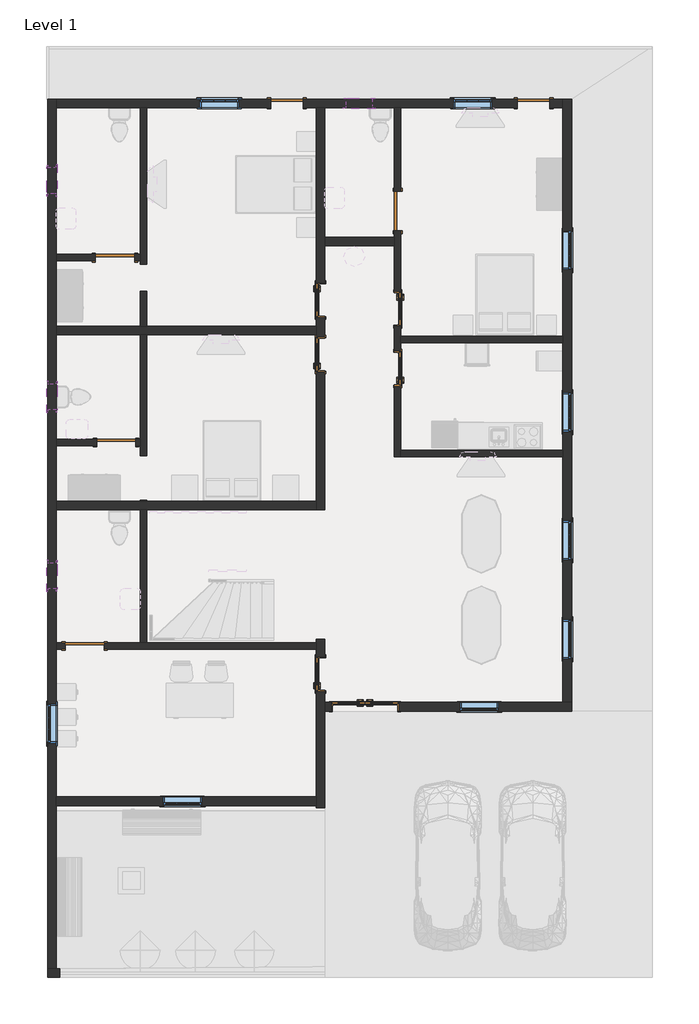
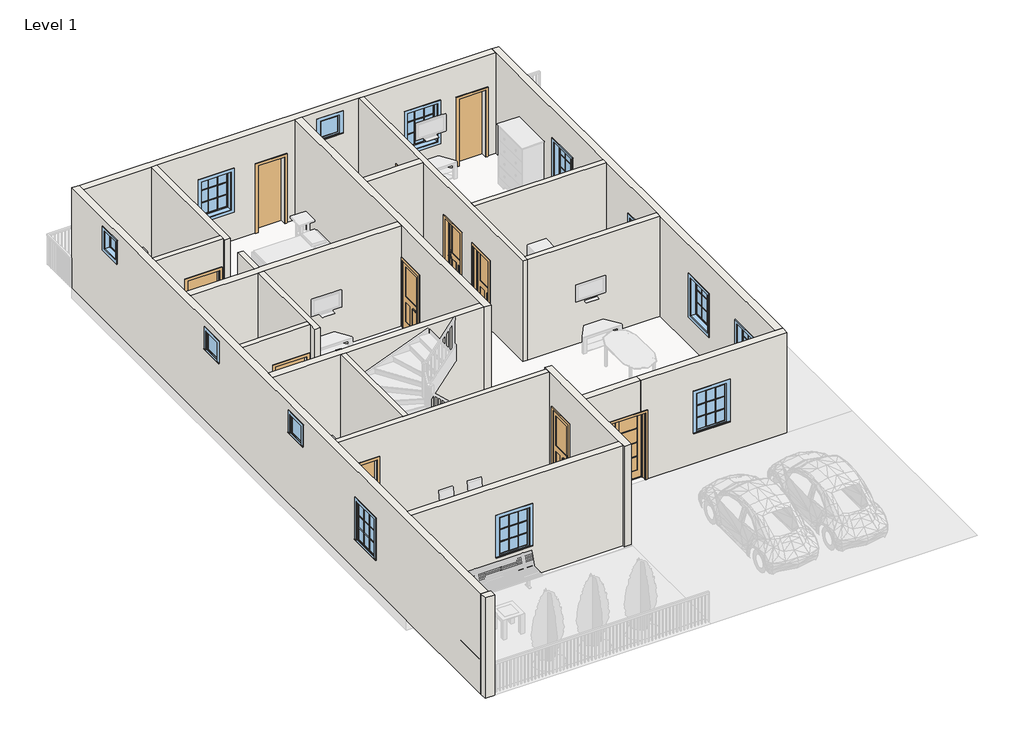
# One storey, part 1 of 4: 22 walls, 13 windows, 12 doors.
"""IFC4 building model written with IfcOpenShell, lengths in millimetres."""

from ifc_helpers import new_model, si_unit, frame, origin, origin_with_axes, place, context, project, spatial, polyline, outline, extrude, faceted_brep, transform, mapped, element, save
from components import door_7e6851c9, door_f50bbf81, door_cdf9d6cc, door_ce1fc124, door_b03bd389, door_fadea3f2, door_16372e1c, door_686f89d2, window_29c06734, window_e41d21a6

model = new_model("IFC4")

# Units and contexts
model_context = context("Model", 3, world=origin())
ifc_project = project(units=[si_unit("LENGTHUNIT", "METRE", prefix="MILLI")], contexts=[model_context])

# Site, building, storey
site = spatial("IfcSite", under=ifc_project)
building = spatial("IfcBuilding", under=site)
storey = spatial("IfcBuildingStorey", under=building, Name="Level 1", Elevation=0.0)

# Doors
placement = place(None, origin())
door_shape = door_7e6851c9(model_context)
element("IfcDoor", 1, ObjectType="30\" x 80\"", at=placement, inside=storey, context=model_context, shape_type="MappedRepresentation", body=[
    mapped(door_shape, transform((831.023647, -4225.8011892, 0.0), x_axis=(0.0, -1.0, 0.0), y_axis=(1.0, 0.0, 0.0), z_axis=(0.0, 0.0, 1.0))),
])
element("IfcDoor", 2, ObjectType="30\" x 80\"", at=placement, inside=storey, context=model_context, shape_type="MappedRepresentation", body=[
    mapped(door_shape, transform((831.023647, 3241.7988108, 0.0), x_axis=(0.0, -1.0, 0.0), y_axis=(1.0, 0.0, 0.0), z_axis=(0.0, 0.0, 1.0))),
])
door_2_shape = door_f50bbf81(model_context)
element("IfcDoor", 3, ObjectType="30\" x 80\"", at=placement, inside=storey, context=model_context, shape_type="MappedRepresentation", body=[
    mapped(door_2_shape, transform((831.023647, 4511.7988108, 0.0), x_axis=(0.0, 1.0, 0.0), y_axis=(-1.0, 0.0, 0.0), z_axis=(0.0, 0.0, 1.0))),
])
door_3_shape = door_cdf9d6cc(model_context)
element("IfcDoor", 4, ObjectType="30\" x 80\"", at=placement, inside=storey, context=model_context, shape_type="MappedRepresentation", body=[
    mapped(door_3_shape, transform((2640.773647, 2911.5988108, 0.0), x_axis=(0.0, -1.0, 0.0), y_axis=(1.0, 0.0, 0.0), z_axis=(0.0, 0.0, 1.0))),
])
door_4_shape = door_ce1fc124(model_context)
element("IfcDoor", 5, ObjectType="30\" x 80\"", at=placement, inside=storey, context=model_context, shape_type="MappedRepresentation", body=[
    mapped(door_4_shape, transform((2640.773647, 4308.5988108, 0.0), x_axis=(0.0, 1.0, 0.0), y_axis=(-1.0, 0.0, 0.0), z_axis=(0.0, 0.0, 1.0))),
])
door_5_shape = door_b03bd389(model_context)
element("IfcDoor", 6, ObjectType="Door-Exterior-Double-Full Glass-Wood_Clad : 60\" x 80\"", at=placement, inside=storey, context=model_context, shape_type="MappedRepresentation", body=[
    mapped(door_5_shape, transform((1875.598647, -4984.6261892, 0.0), x_axis=(1.0, 0.0, 0.0), y_axis=(0.0, 1.0, 0.0), z_axis=(0.0, 0.0, 1.0))),
])
door_6_shape = door_fadea3f2(model_context)
element("IfcDoor", 7, ObjectType="Single-Flush : 30\" x 80\"", at=placement, inside=storey, context=model_context, shape_type="MappedRepresentation", body=[
    mapped(door_6_shape, transform((46.798647, 9109.1988108, 0.0), x_axis=(1.0, 0.0, 0.0), y_axis=(0.0, 1.0, 0.0), z_axis=(0.0, 0.0, 1.0))),
])
element("IfcDoor", 8, ObjectType="Single-Flush : 30\" x 80\"", at=placement, inside=storey, context=model_context, shape_type="MappedRepresentation", body=[
    mapped(door_6_shape, transform((5812.598647, 9109.1988108, 0.0), x_axis=(1.0, 0.0, 0.0), y_axis=(0.0, 1.0, 0.0), z_axis=(0.0, 0.0, 1.0))),
])
door_7_shape = door_16372e1c(model_context)
element("IfcDoor", 9, ObjectType="Single-Flush : 36\" x 84\"", at=placement, inside=storey, context=model_context, shape_type="MappedRepresentation", body=[
    mapped(door_7_shape, transform((-3966.401353, 5502.3988108, 0.0), x_axis=(1.0, 0.0, 0.0), y_axis=(0.0, 1.0, 0.0), z_axis=(0.0, 0.0, 1.0))),
])
element("IfcDoor", 10, ObjectType="Single-Flush : 36\" x 84\"", at=placement, inside=storey, context=model_context, shape_type="MappedRepresentation", body=[
    mapped(door_7_shape, transform((-3941.001353, 1184.3988108, 0.0), x_axis=(1.0, 0.0, 0.0), y_axis=(0.0, 1.0, 0.0), z_axis=(0.0, 0.0, 1.0))),
])
door_8_shape = door_686f89d2(model_context)
element("IfcDoor", 11, ObjectType="Single-Flush : 36\" x 84\"", at=placement, inside=storey, context=model_context, shape_type="MappedRepresentation", body=[
    mapped(door_8_shape, transform((2637.598647, 6594.5988108, 0.0), x_axis=(0.0, -1.0, 0.0), y_axis=(1.0, 0.0, 0.0), z_axis=(0.0, 0.0, 1.0))),
])
element("IfcDoor", 12, ObjectType="Single-Flush : 36\" x 84\"", at=placement, inside=storey, context=model_context, shape_type="MappedRepresentation", body=[
    mapped(door_8_shape, transform((-4677.601353, -3565.4011892, 0.0), x_axis=(-1.0, 0.0, 0.0), y_axis=(0.0, -1.0, 0.0), z_axis=(0.0, 0.0, 1.0))),
])

# Walls
element("IfcWall", 13, ObjectType="Generic - 8\"", at=placement, inside=storey, context=model_context, shape_type="Brep", body=[
    faceted_brep([(-5338.001353, -11109.2011892, 0.0), (-5338.001353, -7299.2011892, 0.0), (-5338.001353, -7096.0011892, 0.0), (-5338.001353, -3641.6011892, 0.0), (-5338.001353, -3489.2011892, 0.0), (-5338.001353, -390.4011892, 0.0), (-5338.001353, -187.2011892, 0.0), (-5338.001353, 1108.1988108, 0.0), (-5338.001353, 1260.5988108, 0.0), (-5338.001353, 3698.9988108, 0.0), (-5338.001353, 3902.1988108, 0.0), (-5338.001353, 5426.1988108, 0.0), (-5338.001353, 5578.5988108, 0.0), (-5338.001353, 9007.5988108, 0.0), (-5338.001353, 9210.7988108, 0.0), (-5338.001353, 9210.7988108, 3048.0), (-5338.001353, 9007.5988108, 3048.0), (-5338.001353, 5578.5988108, 3048.0), (-5338.001353, 5426.1988108, 3048.0), (-5338.001353, 3902.1988108, 3048.0), (-5338.001353, 3698.9988108, 3048.0), (-5338.001353, 1260.5988108, 3048.0), (-5338.001353, 1108.1988108, 3048.0), (-5338.001353, -187.2011892, 3048.0), (-5338.001353, -390.4011892, 3048.0), (-5338.001353, -3489.2011892, 3048.0), (-5338.001353, -3641.6011892, 3048.0), (-5338.001353, -7096.0011892, 3048.0), (-5338.001353, -7299.2011892, 3048.0), (-5338.001353, -11109.2011892, 3048.0), (-5338.001353, -4924.3011892, 2133.6), (-5338.001353, -4924.3011892, 914.4), (-5338.001353, -5838.7011892, 914.4), (-5338.001353, -5838.7011892, 2133.6), (-5338.001353, -1622.3011892, 2768.6), (-5338.001353, -1622.3011892, 2159.0), (-5338.001353, -2231.9011892, 2159.0), (-5338.001353, -2231.9011892, 2768.6), (-5338.001353, 2555.9988108, 2768.6), (-5338.001353, 2555.9988108, 2159.0), (-5338.001353, 1946.3988108, 2159.0), (-5338.001353, 1946.3988108, 2768.6), (-5338.001353, 7000.9988108, 2768.6), (-5338.001353, 7610.5988108, 2768.6), (-5338.001353, 7610.5988108, 2159.0), (-5338.001353, 7000.9988108, 2159.0), (-5541.201353, -11109.2011892, 0.0), (-5541.201353, -11109.2011892, 3048.0), (-5541.201353, 9210.7988108, 3048.0), (-5541.201353, 9210.7988108, 0.0), (-5541.201353, -4924.3011892, 2133.6), (-5541.201353, -5838.7011892, 2133.6), (-5541.201353, -5838.7011892, 914.4), (-5541.201353, -4924.3011892, 914.4), (-5541.201353, -1622.3011892, 2768.6), (-5541.201353, -2231.9011892, 2768.6), (-5541.201353, -2231.9011892, 2159.0), (-5541.201353, -1622.3011892, 2159.0), (-5541.201353, 2555.9988108, 2768.6), (-5541.201353, 1946.3988108, 2768.6), (-5541.201353, 1946.3988108, 2159.0), (-5541.201353, 2555.9988108, 2159.0), (-5541.201353, 7000.9988108, 2768.6), (-5541.201353, 7000.9988108, 2159.0), (-5541.201353, 7610.5988108, 2159.0), (-5541.201353, 7610.5988108, 2768.6)], [[[0, 1, 2, 3, 4, 5, 6, 7, 8, 9, 10, 11, 12, 13, 14, 15, 16, 17, 18, 19, 20, 21, 22, 23, 24, 25, 26, 27, 28, 29], [30, 31, 32, 33], [34, 35, 36, 37], [38, 39, 40, 41], [42, 43, 44, 45]], [[46, 47, 48, 49], [50, 51, 52, 53], [54, 55, 56, 57], [58, 59, 60, 61], [62, 63, 64, 65]], [[14, 13, 12, 11, 10, 9, 8, 7, 6, 5, 4, 3, 2, 1, 0, 46, 49]], [[29, 28, 27, 26, 25, 24, 23, 22, 21, 20, 19, 18, 17, 16, 15, 48, 47]], [[0, 29, 47, 46]], [[15, 14, 49, 48]], [[31, 30, 50, 53]], [[32, 31, 53, 52]], [[33, 32, 52, 51]], [[30, 33, 51, 50]], [[35, 34, 54, 57]], [[36, 35, 57, 56]], [[37, 36, 56, 55]], [[34, 37, 55, 54]], [[39, 38, 58, 61]], [[40, 39, 61, 60]], [[41, 40, 60, 59]], [[38, 41, 59, 58]], [[63, 62, 42, 45]], [[64, 63, 45, 44]], [[65, 64, 44, 43]], [[62, 65, 43, 42]]]),
])
element("IfcWall", 14, ObjectType="Generic - 8\"", at=placement, inside=storey, context=model_context, shape_type="Brep", body=[
    faceted_brep([(6701.598647, -4886.2011892, 0.0), (6701.598647, 9210.7988108, 0.0), (6701.598647, 9210.7988108, 3048.0), (6701.598647, -4886.2011892, 3048.0), (6701.598647, 5222.9988108, 2133.6), (6701.598647, 6137.3988108, 2133.6), (6701.598647, 6137.3988108, 914.4), (6701.598647, 5222.9988108, 914.4), (6701.598647, 1438.3988108, 2133.6), (6701.598647, 2352.7988108, 2133.6), (6701.598647, 2352.7988108, 914.4), (6701.598647, 1438.3988108, 914.4), (6701.598647, -1558.8011892, 2133.6), (6701.598647, -644.4011892, 2133.6), (6701.598647, -644.4011892, 914.4), (6701.598647, -1558.8011892, 914.4), (6701.598647, -3870.2011892, 2133.6), (6701.598647, -2955.8011892, 2133.6), (6701.598647, -2955.8011892, 914.4), (6701.598647, -3870.2011892, 914.4), (6498.398647, -4886.2011892, 0.0), (6498.398647, -4886.2011892, 3048.0), (6498.398647, 854.1988108, 3048.0), (6498.398647, 1006.5988108, 3048.0), (6498.398647, 3521.1988108, 3048.0), (6498.398647, 3673.5988108, 3048.0), (6498.398647, 9007.5988108, 3048.0), (6498.398647, 9210.7988108, 3048.0), (6498.398647, 9210.7988108, 0.0), (6498.398647, 9007.5988108, 0.0), (6498.398647, 3673.5988108, 0.0), (6498.398647, 3521.1988108, 0.0), (6498.398647, 1006.5988108, 0.0), (6498.398647, 854.1988108, 0.0), (6498.398647, 5222.9988108, 2133.6), (6498.398647, 5222.9988108, 914.4), (6498.398647, 6137.3988108, 914.4), (6498.398647, 6137.3988108, 2133.6), (6498.398647, 1438.3988108, 2133.6), (6498.398647, 1438.3988108, 914.4), (6498.398647, 2352.7988108, 914.4), (6498.398647, 2352.7988108, 2133.6), (6498.398647, -1558.8011892, 2133.6), (6498.398647, -1558.8011892, 914.4), (6498.398647, -644.4011892, 914.4), (6498.398647, -644.4011892, 2133.6), (6498.398647, -3870.2011892, 2133.6), (6498.398647, -3870.2011892, 914.4), (6498.398647, -2955.8011892, 914.4), (6498.398647, -2955.8011892, 2133.6)], [[[0, 1, 2, 3], [4, 5, 6, 7], [8, 9, 10, 11], [12, 13, 14, 15], [16, 17, 18, 19]], [[20, 21, 22, 23, 24, 25, 26, 27, 28, 29, 30, 31, 32, 33], [34, 35, 36, 37], [38, 39, 40, 41], [42, 43, 44, 45], [46, 47, 48, 49]], [[1, 0, 20, 33, 32, 31, 30, 29, 28]], [[3, 2, 27, 26, 25, 24, 23, 22, 21]], [[2, 1, 28, 27]], [[0, 3, 21, 20]], [[35, 34, 4, 7]], [[36, 35, 7, 6]], [[37, 36, 6, 5]], [[34, 37, 5, 4]], [[39, 38, 8, 11]], [[40, 39, 11, 10]], [[41, 40, 10, 9]], [[38, 41, 9, 8]], [[43, 42, 12, 15]], [[44, 43, 15, 14]], [[45, 44, 14, 13]], [[42, 45, 13, 12]], [[47, 46, 16, 19]], [[48, 47, 19, 18]], [[49, 48, 18, 17]], [[46, 49, 17, 16]]]),
])
element("IfcWall", 15, ObjectType="Generic - 8\"", at=placement, inside=storey, context=model_context, shape_type="Brep", body=[
    faceted_brep([(6498.398647, 9210.7988108, 0.0), (6193.598647, 9210.7988108, 0.0), (6193.598647, 9210.7988108, 2032.0), (5431.598647, 9210.7988108, 2032.0), (5431.598647, 9210.7988108, 0.0), (427.798647, 9210.7988108, 0.0), (427.798647, 9210.7988108, 2032.0), (-334.201353, 9210.7988108, 2032.0), (-334.201353, 9210.7988108, 0.0), (-5338.001353, 9210.7988108, 0.0), (-5338.001353, 9210.7988108, 3048.0), (6498.398647, 9210.7988108, 3048.0), (-1070.801353, 9210.7988108, 2133.6), (-1985.201353, 9210.7988108, 2133.6), (-1985.201353, 9210.7988108, 914.4), (-1070.801353, 9210.7988108, 914.4), (4847.398647, 9210.7988108, 2133.6), (3932.998647, 9210.7988108, 2133.6), (3932.998647, 9210.7988108, 914.4), (4847.398647, 9210.7988108, 914.4), (1431.098647, 9210.7988108, 2768.6), (1431.098647, 9210.7988108, 2159.0), (2040.698647, 9210.7988108, 2159.0), (2040.698647, 9210.7988108, 2768.6), (6193.598647, 9007.5988108, 2032.0), (6193.598647, 9007.5988108, 0.0), (6498.398647, 9007.5988108, 0.0), (6498.398647, 9007.5988108, 3048.0), (2713.798647, 9007.5988108, 3048.0), (2561.398647, 9007.5988108, 3048.0), (935.798647, 9007.5988108, 3048.0), (732.598647, 9007.5988108, 3048.0), (-3229.801353, 9007.5988108, 3048.0), (-3382.201353, 9007.5988108, 3048.0), (-5338.001353, 9007.5988108, 3048.0), (-5338.001353, 9007.5988108, 0.0), (-3382.201353, 9007.5988108, 0.0), (-3229.801353, 9007.5988108, 0.0), (-334.201353, 9007.5988108, 0.0), (-334.201353, 9007.5988108, 2032.0), (427.798647, 9007.5988108, 2032.0), (427.798647, 9007.5988108, 0.0), (732.598647, 9007.5988108, 0.0), (935.798647, 9007.5988108, 0.0), (2561.398647, 9007.5988108, 0.0), (2713.798647, 9007.5988108, 0.0), (5431.598647, 9007.5988108, 0.0), (5431.598647, 9007.5988108, 2032.0), (-1070.801353, 9007.5988108, 2133.6), (-1070.801353, 9007.5988108, 914.4), (-1985.201353, 9007.5988108, 914.4), (-1985.201353, 9007.5988108, 2133.6), (4847.398647, 9007.5988108, 2133.6), (4847.398647, 9007.5988108, 914.4), (3932.998647, 9007.5988108, 914.4), (3932.998647, 9007.5988108, 2133.6), (1431.098647, 9007.5988108, 2768.6), (2040.698647, 9007.5988108, 2768.6), (2040.698647, 9007.5988108, 2159.0), (1431.098647, 9007.5988108, 2159.0)], [[[0, 1, 2, 3, 4, 5, 6, 7, 8, 9, 10, 11], [12, 13, 14, 15], [16, 17, 18, 19], [20, 21, 22, 23]], [[24, 25, 26, 27, 28, 29, 30, 31, 32, 33, 34, 35, 36, 37, 38, 39, 40, 41, 42, 43, 44, 45, 46, 47], [48, 49, 50, 51], [52, 53, 54, 55], [56, 57, 58, 59]], [[38, 37, 36, 35, 9, 8]], [[26, 25, 1, 0]], [[46, 45, 44, 43, 42, 41, 5, 4]], [[11, 10, 34, 33, 32, 31, 30, 29, 28, 27]], [[10, 9, 35, 34]], [[0, 11, 27, 26]], [[49, 48, 12, 15]], [[50, 49, 15, 14]], [[51, 50, 14, 13]], [[48, 51, 13, 12]], [[53, 52, 16, 19]], [[54, 53, 19, 18]], [[55, 54, 18, 17]], [[52, 55, 17, 16]], [[21, 20, 56, 59]], [[22, 21, 59, 58]], [[23, 22, 58, 57]], [[20, 23, 57, 56]], [[6, 5, 41, 40]], [[7, 6, 40, 39]], [[8, 7, 39, 38]], [[2, 1, 25, 24]], [[3, 2, 24, 47]], [[4, 3, 47, 46]]]),
])
element("IfcWall", 16, ObjectType="Generic - 8\"", at=placement, inside=storey, context=model_context, shape_type="SweptSolid", body=[
    extrude(outline(polyline([(0.0, -5338.001353), (0.0, 732.598647), (3048.0, 732.598647), (3048.0, -5338.001353), (0.0, -5338.001353)]), holes=[polyline([(2133.6, -2848.801353), (2133.6, -1934.401353), (914.4, -1934.401353), (914.4, -2848.801353), (2133.6, -2848.801353)])]), frame((0.0, -7299.2011892, 0.0), z_axis=(0.0, 1.0, 0.0), x_axis=(0.0, 0.0, 1.0)), (0.0, 0.0, 1.0), 203.2),
])
element("IfcWall", 17, ObjectType="Generic - 8\"", at=placement, inside=storey, context=model_context, shape_type="Brep", body=[
    faceted_brep([(935.798647, -3413.0011892, 0.0), (935.798647, -3413.0011892, 3048.0), (935.798647, -4886.2011892, 3048.0), (935.798647, -5089.4011892, 3048.0), (935.798647, -7350.0011892, 3048.0), (935.798647, -7350.0011892, 0.0), (935.798647, -5089.4011892, 0.0), (935.798647, -4886.2011892, 0.0), (935.798647, -4632.2011892, 0.0), (935.798647, -4632.2011892, 2057.4), (935.798647, -3819.4011892, 2057.4), (935.798647, -3819.4011892, 0.0), (732.598647, -3413.0011892, 3048.0), (732.598647, -3413.0011892, 0.0), (732.598647, -3489.2011892, 0.0), (732.598647, -3641.6011892, 0.0), (732.598647, -3819.4011892, 0.0), (732.598647, -3819.4011892, 2057.4), (732.598647, -4632.2011892, 2057.4), (732.598647, -4632.2011892, 0.0), (732.598647, -7096.0011892, 0.0), (732.598647, -7299.2011892, 0.0), (732.598647, -7350.0011892, 0.0), (732.598647, -7350.0011892, 3048.0), (732.598647, -7299.2011892, 3048.0), (732.598647, -7096.0011892, 3048.0), (732.598647, -3641.6011892, 3048.0), (732.598647, -3489.2011892, 3048.0)], [[[0, 1, 2, 3, 4, 5, 6, 7, 8, 9, 10, 11]], [[12, 13, 14, 15, 16, 17, 18, 19, 20, 21, 22, 23, 24, 25, 26, 27]], [[13, 0, 11, 16, 15, 14]], [[5, 22, 21, 20, 19, 8, 7, 6]], [[1, 0, 13, 12]], [[4, 3, 2, 1, 12, 27, 26, 25, 24, 23]], [[5, 4, 23, 22]], [[18, 9, 8, 19]], [[9, 18, 17, 10]], [[10, 17, 16, 11]]]),
])
element("IfcWall", 18, ObjectType="Generic - 8\"", at=placement, inside=storey, context=model_context, shape_type="Brep", body=[
    faceted_brep([(732.598647, -187.2011892, 0.0), (-3229.801353, -187.2011892, 0.0), (-3382.201353, -187.2011892, 0.0), (-5338.001353, -187.2011892, 0.0), (-5338.001353, -187.2011892, 3048.0), (-3382.201353, -187.2011892, 3048.0), (-3229.801353, -187.2011892, 3048.0), (732.598647, -187.2011892, 3048.0), (732.598647, -390.4011892, 0.0), (732.598647, -390.4011892, 3048.0), (-3229.801353, -390.4011892, 3048.0), (-3382.201353, -390.4011892, 3048.0), (-5338.001353, -390.4011892, 3048.0), (-5338.001353, -390.4011892, 0.0), (-3382.201353, -390.4011892, 0.0), (-3229.801353, -390.4011892, 0.0)], [[[0, 1, 2, 3, 4, 5, 6, 7]], [[8, 9, 10, 11, 12, 13, 14, 15]], [[3, 2, 1, 0, 8, 15, 14, 13]], [[7, 6, 5, 4, 12, 11, 10, 9]], [[4, 3, 13, 12]], [[0, 7, 9, 8]]]),
])
element("IfcWall", 19, ObjectType="Generic - 8\"", at=placement, inside=storey, context=model_context, shape_type="Brep", body=[
    faceted_brep([(732.598647, 3902.1988108, 0.0), (-3229.801353, 3902.1988108, 0.0), (-3382.201353, 3902.1988108, 0.0), (-5338.001353, 3902.1988108, 0.0), (-5338.001353, 3902.1988108, 3048.0), (-3382.201353, 3902.1988108, 3048.0), (-3229.801353, 3902.1988108, 3048.0), (732.598647, 3902.1988108, 3048.0), (732.598647, 3698.9988108, 0.0), (732.598647, 3698.9988108, 3048.0), (-3229.801353, 3698.9988108, 3048.0), (-3382.201353, 3698.9988108, 3048.0), (-5338.001353, 3698.9988108, 3048.0), (-5338.001353, 3698.9988108, 0.0), (-3382.201353, 3698.9988108, 0.0), (-3229.801353, 3698.9988108, 0.0)], [[[0, 1, 2, 3, 4, 5, 6, 7]], [[8, 9, 10, 11, 12, 13, 14, 15]], [[3, 2, 1, 0, 8, 15, 14, 13]], [[7, 6, 5, 4, 12, 11, 10, 9]], [[4, 3, 13, 12]], [[0, 7, 9, 8]]]),
])
element("IfcWall", 20, ObjectType="Generic - 8\"", at=placement, inside=storey, context=model_context, shape_type="SweptSolid", body=[
    extrude(outline(polyline([(3048.0, 2510.598647), (3048.0, 935.798647), (0.0, 935.798647), (0.0, 1088.198647), (2057.4, 1088.198647), (2057.4, 2510.598647), (3048.0, 2510.598647)])), frame((0.0, -5089.4011892, 0.0), z_axis=(0.0, 1.0, 0.0), x_axis=(0.0, 0.0, 1.0)), (0.0, 0.0, 1.0), 203.2),
])
element("IfcWall", 21, ObjectType="Generic - 8\"", at=placement, inside=storey, context=model_context, shape_type="SweptSolid", body=[
    extrude(outline(polyline([(935.798647, 5984.9988108), (2561.398647, 5984.9988108), (2561.398647, 5781.7988108), (935.798647, 5781.7988108), (935.798647, 5984.9988108)])), origin_with_axes(), (0.0, 0.0, 1.0), 3048.0),
])
element("IfcWall", 22, ObjectType="Generic - 8\"", at=placement, inside=storey, context=model_context, shape_type="Brep", body=[
    faceted_brep([(2510.598647, -4886.2011892, 3048.0), (6498.398647, -4886.2011892, 3048.0), (6701.598647, -4886.2011892, 3048.0), (6701.598647, -4886.2011892, 0.0), (6498.398647, -4886.2011892, 0.0), (2662.998647, -4886.2011892, 0.0), (2662.998647, -4886.2011892, 2057.4), (2510.598647, -4886.2011892, 2057.4), (4085.398647, -4886.2011892, 2133.6), (4085.398647, -4886.2011892, 914.4), (4999.798647, -4886.2011892, 914.4), (4999.798647, -4886.2011892, 2133.6), (6701.598647, -5089.4011892, 3048.0), (2510.598647, -5089.4011892, 3048.0), (2510.598647, -5089.4011892, 2057.4), (2662.998647, -5089.4011892, 2057.4), (2662.998647, -5089.4011892, 0.0), (6701.598647, -5089.4011892, 0.0), (4085.398647, -5089.4011892, 2133.6), (4999.798647, -5089.4011892, 2133.6), (4999.798647, -5089.4011892, 914.4), (4085.398647, -5089.4011892, 914.4)], [[[0, 1, 2, 3, 4, 5, 6, 7], [8, 9, 10, 11]], [[12, 13, 14, 15, 16, 17], [18, 19, 20, 21]], [[3, 17, 16, 5, 4]], [[13, 0, 7, 14]], [[2, 1, 0, 13, 12]], [[3, 2, 12, 17]], [[15, 6, 5, 16]], [[6, 15, 14, 7]], [[9, 8, 18, 21]], [[10, 9, 21, 20]], [[11, 10, 20, 19]], [[8, 11, 19, 18]]]),
])
element("IfcWall", 23, ObjectType="Generic - 8\"", at=placement, inside=storey, context=model_context, shape_type="Brep", body=[
    faceted_brep([(935.798647, 9007.5988108, 3048.0), (935.798647, 5984.9988108, 3048.0), (935.798647, 5781.7988108, 3048.0), (935.798647, -390.4011892, 3048.0), (935.798647, -390.4011892, 0.0), (935.798647, 2835.3988108, 0.0), (935.798647, 2835.3988108, 2057.4), (935.798647, 3648.1988108, 2057.4), (935.798647, 3648.1988108, 0.0), (935.798647, 4105.3988108, 0.0), (935.798647, 4105.3988108, 2057.4), (935.798647, 4918.1988108, 2057.4), (935.798647, 4918.1988108, 0.0), (935.798647, 5781.7988108, 0.0), (935.798647, 5984.9988108, 0.0), (935.798647, 9007.5988108, 0.0), (732.598647, -390.4011892, 3048.0), (732.598647, -187.2011892, 3048.0), (732.598647, 3698.9988108, 3048.0), (732.598647, 3902.1988108, 3048.0), (732.598647, 9007.5988108, 3048.0), (732.598647, 9007.5988108, 0.0), (732.598647, 4918.1988108, 0.0), (732.598647, 4918.1988108, 2057.4), (732.598647, 4105.3988108, 2057.4), (732.598647, 4105.3988108, 0.0), (732.598647, 3902.1988108, 0.0), (732.598647, 3698.9988108, 0.0), (732.598647, 3648.1988108, 0.0), (732.598647, 3648.1988108, 2057.4), (732.598647, 2835.3988108, 2057.4), (732.598647, 2835.3988108, 0.0), (732.598647, -187.2011892, 0.0), (732.598647, -390.4011892, 0.0)], [[[0, 1, 2, 3, 4, 5, 6, 7, 8, 9, 10, 11, 12, 13, 14, 15]], [[16, 17, 18, 19, 20, 21, 22, 23, 24, 25, 26, 27, 28, 29, 30, 31, 32, 33]], [[21, 15, 14, 13, 12, 22]], [[4, 33, 32, 31, 5]], [[25, 9, 8, 28, 27, 26]], [[3, 2, 1, 0, 20, 19, 18, 17, 16]], [[0, 15, 21, 20]], [[4, 3, 16, 33]], [[11, 23, 22, 12]], [[23, 11, 10, 24]], [[24, 10, 9, 25]], [[30, 6, 5, 31]], [[6, 30, 29, 7]], [[7, 29, 28, 8]]]),
])
element("IfcWall", 24, ObjectType="Generic - 8\"", at=placement, inside=storey, context=model_context, shape_type="Brep", body=[
    faceted_brep([(-5261.801353, -11109.2011892, 0.0), (-5338.001353, -11109.2011892, 0.0), (-5541.201353, -11109.2011892, 0.0), (-5541.201353, -11109.2011892, 3048.0), (-5338.001353, -11109.2011892, 3048.0), (-5261.801353, -11109.2011892, 3048.0), (-5261.801353, -11312.4011892, 0.0), (-5261.801353, -11312.4011892, 3048.0), (-5541.201353, -11312.4011892, 3048.0), (-5541.201353, -11312.4011892, 0.0)], [[[0, 1, 2, 3, 4, 5]], [[6, 7, 8, 9]], [[2, 1, 0, 6, 9]], [[5, 4, 3, 8, 7]], [[0, 5, 7, 6]], [[3, 2, 9, 8]]]),
])
element("IfcWall", 25, ObjectType="Inner wall", at=placement, inside=storey, context=model_context, shape_type="Brep", body=[
    faceted_brep([(2561.398647, 854.1988108, 3048.0), (2561.398647, 5781.7988108, 3048.0), (2561.398647, 5984.9988108, 3048.0), (2561.398647, 9007.5988108, 3048.0), (2561.398647, 9007.5988108, 0.0), (2561.398647, 7051.7988108, 0.0), (2561.398647, 7051.7988108, 2133.6), (2561.398647, 6137.3988108, 2133.6), (2561.398647, 6137.3988108, 0.0), (2561.398647, 5984.9988108, 0.0), (2561.398647, 5781.7988108, 0.0), (2561.398647, 4714.9988108, 0.0), (2561.398647, 4714.9988108, 2057.4), (2561.398647, 3902.1988108, 2057.4), (2561.398647, 3902.1988108, 0.0), (2561.398647, 3317.9988108, 0.0), (2561.398647, 3317.9988108, 2057.4), (2561.398647, 2505.1988108, 2057.4), (2561.398647, 2505.1988108, 0.0), (2561.398647, 854.1988108, 0.0), (2713.798647, 9007.5988108, 3048.0), (2713.798647, 3673.5988108, 3048.0), (2713.798647, 3521.1988108, 3048.0), (2713.798647, 1006.5988108, 3048.0), (2713.798647, 854.1988108, 3048.0), (2713.798647, 854.1988108, 0.0), (2713.798647, 1006.5988108, 0.0), (2713.798647, 2505.1988108, 0.0), (2713.798647, 2505.1988108, 2057.4), (2713.798647, 3317.9988108, 2057.4), (2713.798647, 3317.9988108, 0.0), (2713.798647, 3521.1988108, 0.0), (2713.798647, 3673.5988108, 0.0), (2713.798647, 3902.1988108, 0.0), (2713.798647, 3902.1988108, 2057.4), (2713.798647, 4714.9988108, 2057.4), (2713.798647, 4714.9988108, 0.0), (2713.798647, 6137.3988108, 0.0), (2713.798647, 6137.3988108, 2133.6), (2713.798647, 7051.7988108, 2133.6), (2713.798647, 7051.7988108, 0.0), (2713.798647, 9007.5988108, 0.0)], [[[0, 1, 2, 3, 4, 5, 6, 7, 8, 9, 10, 11, 12, 13, 14, 15, 16, 17, 18, 19]], [[20, 21, 22, 23, 24, 25, 26, 27, 28, 29, 30, 31, 32, 33, 34, 35, 36, 37, 38, 39, 40, 41]], [[4, 41, 40, 5]], [[25, 19, 18, 27, 26]], [[8, 37, 36, 11, 10, 9]], [[30, 15, 14, 33, 32, 31]], [[3, 2, 1, 0, 24, 23, 22, 21, 20]], [[4, 3, 20, 41]], [[0, 19, 25, 24]], [[38, 37, 8, 7]], [[39, 38, 7, 6]], [[40, 39, 6, 5]], [[17, 28, 27, 18]], [[28, 17, 16, 29]], [[29, 16, 15, 30]], [[35, 12, 11, 36]], [[12, 35, 34, 13]], [[13, 34, 33, 14]]]),
])
element("IfcWall", 26, ObjectType="Inner wall", at=placement, inside=storey, context=model_context, shape_type="Brep", body=[
    faceted_brep([(-5134.801353, -3489.2011892, 2133.6), (-5134.801353, -3489.2011892, 0.0), (-5338.001353, -3489.2011892, 0.0), (-5338.001353, -3489.2011892, 3048.0), (-3382.201353, -3489.2011892, 3048.0), (-3229.801353, -3489.2011892, 3048.0), (732.598647, -3489.2011892, 3048.0), (732.598647, -3489.2011892, 0.0), (-3229.801353, -3489.2011892, 0.0), (-3382.201353, -3489.2011892, 0.0), (-4220.401353, -3489.2011892, 0.0), (-4220.401353, -3489.2011892, 2133.6), (-5338.001353, -3641.6011892, 0.0), (-5134.801353, -3641.6011892, 0.0), (-5134.801353, -3641.6011892, 2133.6), (-4220.401353, -3641.6011892, 2133.6), (-4220.401353, -3641.6011892, 0.0), (732.598647, -3641.6011892, 0.0), (732.598647, -3641.6011892, 3048.0), (-5338.001353, -3641.6011892, 3048.0)], [[[0, 1, 2, 3, 4, 5, 6, 7, 8, 9, 10, 11]], [[12, 13, 14, 15, 16, 17, 18, 19]], [[2, 1, 13, 12]], [[10, 9, 8, 7, 17, 16]], [[6, 5, 4, 3, 19, 18]], [[3, 2, 12, 19]], [[7, 6, 18, 17]], [[14, 13, 1, 0]], [[15, 14, 0, 11]], [[16, 15, 11, 10]]]),
])
element("IfcWall", 27, ObjectType="Inner wall", at=placement, inside=storey, context=model_context, shape_type="Brep", body=[
    faceted_brep([(-3382.201353, 9007.5988108, 0.0), (-3382.201353, 5578.5988108, 0.0), (-3382.201353, 5426.1988108, 0.0), (-3382.201353, 5349.9988108, 0.0), (-3382.201353, 5349.9988108, 3048.0), (-3382.201353, 5426.1988108, 3048.0), (-3382.201353, 5578.5988108, 3048.0), (-3382.201353, 9007.5988108, 3048.0), (-3229.801353, 9007.5988108, 0.0), (-3229.801353, 9007.5988108, 3048.0), (-3229.801353, 5349.9988108, 3048.0), (-3229.801353, 5349.9988108, 0.0)], [[[0, 1, 2, 3, 4, 5, 6, 7]], [[8, 9, 10, 11]], [[3, 2, 1, 0, 8, 11]], [[4, 3, 11, 10]], [[7, 6, 5, 4, 10, 9]], [[0, 7, 9, 8]]]),
])
element("IfcWall", 28, ObjectType="Inner wall", at=placement, inside=storey, context=model_context, shape_type="SweptSolid", body=[
    extrude(outline(polyline([(2713.798647, 1006.5988108), (6498.398647, 1006.5988108), (6498.398647, 854.1988108), (2713.798647, 854.1988108), (2713.798647, 1006.5988108)])), origin_with_axes(), (0.0, 0.0, 1.0), 3048.0),
])
element("IfcWall", 29, ObjectType="Inner wall", at=placement, inside=storey, context=model_context, shape_type="SweptSolid", body=[
    extrude(outline(polyline([(2713.798647, 3673.5988108), (6498.398647, 3673.5988108), (6498.398647, 3521.1988108), (2713.798647, 3521.1988108), (2713.798647, 3673.5988108)])), origin_with_axes(), (0.0, 0.0, 1.0), 3048.0),
])
element("IfcWall", 30, ObjectType="Inner wall", at=placement, inside=storey, context=model_context, shape_type="SweptSolid", body=[
    extrude(outline(polyline([(-3229.801353, -390.4011892), (-3229.801353, -3489.2011892), (-3382.201353, -3489.2011892), (-3382.201353, -390.4011892), (-3229.801353, -390.4011892)])), origin_with_axes(), (0.0, 0.0, 1.0), 3048.0),
])
element("IfcWall", 31, ObjectType="Inner wall", at=placement, inside=storey, context=model_context, shape_type="SweptSolid", body=[
    extrude(outline(polyline([(3048.0, -3382.201353), (3048.0, -5338.001353), (0.0, -5338.001353), (0.0, -4423.601353), (2133.6, -4423.601353), (2133.6, -3509.201353), (0.0, -3509.201353), (0.0, -3382.201353), (3048.0, -3382.201353)])), frame((0.0, 5426.1988108, 0.0), z_axis=(0.0, 1.0, 0.0), x_axis=(0.0, 0.0, 1.0)), (0.0, 0.0, 1.0), 152.4),
])
element("IfcWall", 32, ObjectType="Inner wall", at=placement, inside=storey, context=model_context, shape_type="SweptSolid", body=[
    extrude(outline(polyline([(2133.6, -3483.801353), (0.0, -3483.801353), (0.0, -3382.201353), (3048.0, -3382.201353), (3048.0, -5338.001353), (0.0, -5338.001353), (0.0, -4398.201353), (2133.6, -4398.201353), (2133.6, -3483.801353)])), frame((0.0, 1108.1988108, 0.0), z_axis=(0.0, 1.0, 0.0), x_axis=(0.0, 0.0, 1.0)), (0.0, 0.0, 1.0), 152.4),
])
element("IfcWall", 33, ObjectType="Inner wall", at=placement, inside=storey, context=model_context, shape_type="Brep", body=[
    faceted_brep([(-3382.201353, 879.5988108, 0.0), (-3382.201353, 879.5988108, 3048.0), (-3382.201353, 1108.1988108, 3048.0), (-3382.201353, 1260.5988108, 3048.0), (-3382.201353, 3698.9988108, 3048.0), (-3382.201353, 3698.9988108, 0.0), (-3382.201353, 1260.5988108, 0.0), (-3382.201353, 1108.1988108, 0.0), (-3229.801353, 879.5988108, 3048.0), (-3229.801353, 879.5988108, 0.0), (-3229.801353, 3698.9988108, 0.0), (-3229.801353, 3698.9988108, 3048.0)], [[[0, 1, 2, 3, 4, 5, 6, 7]], [[8, 9, 10, 11]], [[9, 0, 7, 6, 5, 10]], [[1, 0, 9, 8]], [[1, 8, 11, 4, 3, 2]], [[5, 4, 11, 10]]]),
    faceted_brep([(-3382.201353, 4714.9988108, 3048.0), (-3382.201353, 4714.9988108, 0.0), (-3382.201353, 3902.1988108, 0.0), (-3382.201353, 3902.1988108, 3048.0), (-3229.801353, 4714.9988108, 0.0), (-3229.801353, 4714.9988108, 3048.0), (-3229.801353, 3902.1988108, 3048.0), (-3229.801353, 3902.1988108, 0.0)], [[[0, 1, 2, 3]], [[4, 5, 6, 7]], [[1, 4, 7, 2]], [[5, 0, 3, 6]], [[1, 0, 5, 4]], [[3, 2, 7, 6]]]),
])
element("IfcWall", 34, ObjectType="Inner wall", at=placement, inside=storey, context=model_context, shape_type="SweptSolid", body=[
    extrude(outline(polyline([(-3382.201353, -187.2011892), (-3382.201353, -161.8011892), (-3229.801353, -161.8011892), (-3229.801353, -187.2011892), (-3382.201353, -187.2011892)])), origin_with_axes(), (0.0, 0.0, 1.0), 3048.0),
])

# Windows
window_shape = window_29c06734(model_context)
element("IfcWindow", 35, ObjectType="Casement 3x3 with Trim : 36\" x 48\"", at=placement, inside=storey, context=model_context, shape_type="MappedRepresentation", body=[
    mapped(window_shape, transform((-1528.001353, 9109.1988108, 0.0), x_axis=(1.0, 0.0, 0.0), y_axis=(0.0, 1.0, 0.0), z_axis=(0.0, 0.0, 1.0))),
])
element("IfcWindow", 36, ObjectType="Casement 3x3 with Trim : 36\" x 48\"", at=placement, inside=storey, context=model_context, shape_type="MappedRepresentation", body=[
    mapped(window_shape, transform((4390.198647, 9109.1988108, 0.0), x_axis=(1.0, 0.0, 0.0), y_axis=(0.0, 1.0, 0.0), z_axis=(0.0, 0.0, 1.0))),
])
element("IfcWindow", 37, ObjectType="Casement 3x3 with Trim : 36\" x 48\"", at=placement, inside=storey, context=model_context, shape_type="MappedRepresentation", body=[
    mapped(window_shape, transform((6599.998647, 5680.1988108, 0.0), x_axis=(0.0, -1.0, 0.0), y_axis=(1.0, 0.0, 0.0), z_axis=(0.0, 0.0, 1.0))),
])
element("IfcWindow", 38, ObjectType="Casement 3x3 with Trim : 36\" x 48\"", at=placement, inside=storey, context=model_context, shape_type="MappedRepresentation", body=[
    mapped(window_shape, transform((6599.998647, 1895.5988108, 0.0), x_axis=(0.0, -1.0, 0.0), y_axis=(1.0, 0.0, 0.0), z_axis=(0.0, 0.0, 1.0))),
])
element("IfcWindow", 39, ObjectType="Casement 3x3 with Trim : 36\" x 48\"", at=placement, inside=storey, context=model_context, shape_type="MappedRepresentation", body=[
    mapped(window_shape, transform((6599.998647, -1101.6011892, 0.0), x_axis=(0.0, -1.0, 0.0), y_axis=(1.0, 0.0, 0.0), z_axis=(0.0, 0.0, 1.0))),
])
element("IfcWindow", 40, ObjectType="Casement 3x3 with Trim : 36\" x 48\"", at=placement, inside=storey, context=model_context, shape_type="MappedRepresentation", body=[
    mapped(window_shape, transform((6599.998647, -3413.0011892, 0.0), x_axis=(0.0, -1.0, 0.0), y_axis=(1.0, 0.0, 0.0), z_axis=(0.0, 0.0, 1.0))),
])
element("IfcWindow", 41, ObjectType="Casement 3x3 with Trim : 36\" x 48\"", at=placement, inside=storey, context=model_context, shape_type="MappedRepresentation", body=[
    mapped(window_shape, transform((-2391.601353, -7197.6011892, 0.0), x_axis=(-1.0, 0.0, 0.0), y_axis=(0.0, -1.0, 0.0), z_axis=(0.0, 0.0, 1.0))),
])
element("IfcWindow", 42, ObjectType="Casement 3x3 with Trim : 36\" x 48\"", at=placement, inside=storey, context=model_context, shape_type="MappedRepresentation", body=[
    mapped(window_shape, transform((-5439.601353, -5381.5011892, 0.0), x_axis=(0.0, 1.0, 0.0), y_axis=(-1.0, 0.0, 0.0), z_axis=(0.0, 0.0, 1.0))),
])
element("IfcWindow", 43, ObjectType="Casement 3x3 with Trim : 36\" x 48\"", at=placement, inside=storey, context=model_context, shape_type="MappedRepresentation", body=[
    mapped(window_shape, transform((4542.598647, -4987.8011892, 0.0), x_axis=(-1.0, 0.0, 0.0), y_axis=(0.0, -1.0, 0.0), z_axis=(0.0, 0.0, 1.0))),
])
window_2_shape = window_e41d21a6(model_context)
element("IfcWindow", 44, ObjectType="Transom with Trim : 24\" x 24\"", at=placement, inside=storey, context=model_context, shape_type="MappedRepresentation", body=[
    mapped(window_2_shape, transform((-5439.601353, -1889.0011892, 0.0), x_axis=(0.0, 1.0, 0.0), y_axis=(-1.0, 0.0, 0.0), z_axis=(0.0, 0.0, 1.0))),
])
element("IfcWindow", 45, ObjectType="Transom with Trim : 24\" x 24\"", at=placement, inside=storey, context=model_context, shape_type="MappedRepresentation", body=[
    mapped(window_2_shape, transform((-5439.601353, 2289.2988108, 0.0), x_axis=(0.0, 1.0, 0.0), y_axis=(-1.0, 0.0, 0.0), z_axis=(0.0, 0.0, 1.0))),
])
element("IfcWindow", 46, ObjectType="Transom with Trim : 24\" x 24\"", at=placement, inside=storey, context=model_context, shape_type="MappedRepresentation", body=[
    mapped(window_2_shape, transform((-5439.601353, 7267.6988108, 0.0), x_axis=(0.0, -1.0, 0.0), y_axis=(1.0, 0.0, 0.0), z_axis=(0.0, 0.0, 1.0))),
])
element("IfcWindow", 47, ObjectType="Transom with Trim : 24\" x 24\"", at=placement, inside=storey, context=model_context, shape_type="MappedRepresentation", body=[
    mapped(window_2_shape, transform((1697.798647, 9109.1988108, 0.0), x_axis=(-1.0, 0.0, 0.0), y_axis=(0.0, -1.0, 0.0), z_axis=(0.0, 0.0, 1.0))),
])

save(model, "model.ifc")

# Revit data of these elements
# Type "30\" x 80\""
#   Type Mark = "8"
#   Assembly Code = "B2030100"
#   Analytic Construction = "French door, wood frame with single glass"
#   Top Rail = 0' - 4 3/4"
#   Threshold Offset [instance default] = 0' - 0 1/2"
#   Thickness = 0' - 1 3/8"
#   Thermal Resistance (R) = 1.0696 (h·ft²·°F)/BTU
#   Swing Angle [instance default] = 90.00°
#   Stiles = 0' - 4 3/4"
#   Rough Width = 2' - 8"
#   Rough Height = 6' - 9"
#   Lock Rail = 0' - 7 1/8"
#   Height = 6' - 8"
#   Width = 2' - 6"
#   Heat Transfer Coefficient (U) = 0.9350 BTU/(h·ft²·°F)
#   Door Offset [instance default] = 0' - 0"
#   Bottom Rail = 0' - 9 1/2"
#   Threshold [instance default] = yes
#   Function = 1
#   Exterior Trim [instance default] = yes
#   Trim Material = Cherry
#   Threshold Material = Cherry
#   Panel Material = Cherry
#   Glazing = Glass
#   Frame Material = Cherry
#   Door Handle Material = Aluminum
#   Visual Light Transmittance = 0
#   Solar Heat Gain Coefficient = 0
#   Wall Closure = (empty or 0)
#   Construction Type = (empty or 0)
# Type "Door-Exterior-Double-Full Glass-Wood_Clad : 60\" x 80\""
#   Type Mark = "9"
#   Assembly Code = "B2030100"
#   Analytic Construction = "French door, wood frame with double glass"
#   Top Rail = 0' - 4 11/16"
#   Threshold Offset [instance default] = 0' - 0 1/2"
#   Thickness = 0' - 1 3/8"
#   Thermal Resistance (R) = 1.9158 (h·ft²·°F)/BTU
#   Swing Angle [instance default] = 90.00°
#   Stiles = 0' - 4 3/4"
#   Rough Width = 5' - 2"
#   Rough Height = 6' - 9"
#   Panel Width = 2' - 6"
#   Door Offset [instance default] = 0' - 0"
#   Height = 6' - 8"
#   Width = 5' - 0"
#   Heat Transfer Coefficient (U) = 0.5220 BTU/(h·ft²·°F)
#   Bottom Rail = 0' - 9 1/8"
#   Exterior Trim [instance default] = yes
#   Threshold [instance default] = yes
#   Show Grill [instance default] = yes
#   Function = 1
#   Trim Material = Cherry
#   Threshold Material = Cherry
#   Panel Material = Cherry
#   Glazing = Glass
#   Frame Material = Cherry
#   Door Handle Material = Aluminum
#   Visual Light Transmittance = 0
#   Solar Heat Gain Coefficient = 0
#   Wall Closure = (empty or 0)
#   Construction Type = (empty or 0)
# Type "Single-Flush : 30\" x 80\""
#   Type Mark = "5"
#   Construction Type Id = "MDOOR"
#   Assembly Code = "C1020"
#   Analytic Construction = "Metal"
#   Thickness = 0' - 2"
#   Heat Transfer Coefficient (U) = 0.651978 BTU/(h·ft²·°F)
#   Height = 6' - 8"
#   Trim Projection Ext = 0' - 1"
#   Trim Projection Int = 0' - 1"
#   Trim Width = 0' - 3"
#   Width = 2' - 6"
#   Define Thermal Properties by = 1
#   Door Material = Door - Panel
#   Frame Material = Door - Frame
#   Visual Light Transmittance = 0
#   Solar Heat Gain Coefficient = 0
#   Function = (empty or 0)
#   Wall Closure = (empty or 0)
# Type "Single-Flush : 36\" x 84\""
#   Type Mark = "1"
#   Construction Type Id = "MDOOR"
#   Assembly Code = "C1020"
#   Analytic Construction = "Metal"
#   Thickness = 0' - 2"
#   Heat Transfer Coefficient (U) = 0.651978 BTU/(h·ft²·°F)
#   Height = 7' - 0"
#   Trim Projection Ext = 0' - 1"
#   Trim Projection Int = 0' - 1"
#   Trim Width = 0' - 3"
#   Width = 3' - 0"
#   Define Thermal Properties by = 1
#   Door Material = Door - Panel
#   Frame Material = Door - Frame
#   Visual Light Transmittance = 0
#   Solar Heat Gain Coefficient = 0
#   Function = (empty or 0)
#   Wall Closure = (empty or 0)
# Type "Generic - 8\""
#   Assembly Code = "B2010"
#   Layers, outside or top first: 0' - 8" no material (function 1)
# Type "Inner wall"
#   Assembly Code = "B2010"
#   Layers, outside or top first: 0' - 6" no material (function 1)
# Type "Casement 3x3 with Trim : 36\" x 48\""
#   Type Mark = "10"
#   Construction Type Id = "GSP4R"
#   Assembly Code = "B2020100"
#   Analytic Construction = "1/8 in Pilkington single glazing"
#   Visual Light Transmittance = 0.9
#   Solar Heat Gain Coefficient = 0.78
#   Heat Transfer Coefficient (U) = 0.6496 BTU/(h·ft²·°F)
#   Height = 4' - 0"
#   Default Sill Height = 3' - 0"
#   Trim Projection - Ext. = 0' - 0 1/2"
#   Trim Projection - Int. = 0' - 0 3/4"
#   Trim Width - Exterior = 0' - 3 1/2"
#   Trim Width - Interior = 0' - 3 1/2"
#   Width = 3' - 0"
#   Window Inset = 0' - 0 3/4"
#   Define Thermal Properties by = 1
#   Glass Pane Material = Glass
#   Sash Material = Sash
#   Trim Exterior Material = Trim
#   Trim Interior Material = Trim
#   Wall Closure = (empty or 0)
# Type "Transom with Trim : 24\" x 24\""
#   Type Mark = "13"
#   Construction Type Id = "GSP4R"
#   Assembly Code = "B2020100"
#   Analytic Construction = "1/8 in Pilkington single glazing"
#   Visual Light Transmittance = 0.9
#   Solar Heat Gain Coefficient = 0.78
#   Heat Transfer Coefficient (U) = 0.6496 BTU/(h·ft²·°F)
#   Height = 2' - 0"
#   Default Sill Height = 7' - 1"
#   Trim Projection - Ext. = 0' - 0 1/2"
#   Trim Projection - Int. = 0' - 0 3/4"
#   Trim Width - Exterior = 0' - 3 1/2"
#   Trim Width - Interior = 0' - 3 1/2"
#   Width = 2' - 0"
#   Window Inset = 0' - 0 3/4"
#   Define Thermal Properties by = 1
#   Glass Pane Material = Glass
#   Sash Material = Sash
#   Trim Exterior Material = Trim
#   Trim Interior Material = Trim
#   Wall Closure = (empty or 0)
# Elements 1, 2, 3, 4, 5 (IfcDoor, "30\" x 80\"")
#   Threshold Offset = 0' - 0 1/2"
#   Swing Angle = 90.00°
#   Door Offset = 0' - 0"
#   Threshold = yes
#   Exterior Trim = yes
#   Phase Created = New Construction
#   Materials on its faces: "Cherry", "Aluminum", "Glass"
# Element 6 (IfcDoor, "Door-Exterior-Double-Full Glass-Wood_Clad : 60\" x 80\"")
#   Threshold Offset = 0' - 0 1/2"
#   Swing Angle = 90.00°
#   Door Offset = 0' - 0"
#   Threshold = yes
#   Show Grill = yes
#   Exterior Trim = yes
#   Phase Created = New Construction
#   Materials on its faces: "Cherry", "Aluminum", "Glass"
# Elements 7, 8 (IfcDoor, "Single-Flush : 30\" x 80\"")
#   Phase Created = New Construction
#   Materials on its faces: "Door - Frame", "Door - Panel"
# Elements 9, 10, 11, 12 (IfcDoor, "Single-Flush : 36\" x 84\"")
#   Phase Created = New Construction
#   Materials on its faces: "Door - Frame", "Door - Panel"
# Elements 13, 14, 15, 16, 17, 18, 19, 20, 21, 22, 23, 24 (IfcWall, "Generic - 8\"")
#   Top Offset = 0' - 0"
#   Base Offset = 0' - 0"
#   Unconnected Height = 10' - 0"
#   wall height = 10' - 0"
#   Phase Created = New Construction
#   Base Constraint = Level 1
#   Materials on its faces: "Default Wall"
# Elements 25, 26, 27, 28, 29, 30, 31, 32, 33, 34 (IfcWall, "Inner wall")
#   Top Offset = 0' - 0"
#   Base Offset = 0' - 0"
#   Unconnected Height = 10' - 0"
#   wall height = 10' - 0"
#   Phase Created = New Construction
#   Base Constraint = Level 1
#   Materials on its faces: "Default Wall"
# Element 35 (IfcWindow, "Casement 3x3 with Trim : 36\" x 48\"")
#   Mark = "1"
#   Phase Created = New Construction
#   Materials on its faces: "Sash", "Glass", "Trim"
# Element 36 (IfcWindow, "Casement 3x3 with Trim : 36\" x 48\"")
#   Mark = "2"
#   Phase Created = New Construction
#   Materials on its faces: "Sash", "Glass", "Trim"
# Element 37 (IfcWindow, "Casement 3x3 with Trim : 36\" x 48\"")
#   Mark = "3"
#   Phase Created = New Construction
#   Materials on its faces: "Sash", "Glass", "Trim"
# Element 38 (IfcWindow, "Casement 3x3 with Trim : 36\" x 48\"")
#   Mark = "4"
#   Phase Created = New Construction
#   Materials on its faces: "Sash", "Glass", "Trim"
# Element 39 (IfcWindow, "Casement 3x3 with Trim : 36\" x 48\"")
#   Mark = "5"
#   Phase Created = New Construction
#   Materials on its faces: "Sash", "Glass", "Trim"
# Element 40 (IfcWindow, "Casement 3x3 with Trim : 36\" x 48\"")
#   Mark = "6"
#   Phase Created = New Construction
#   Materials on its faces: "Sash", "Glass", "Trim"
# Element 41 (IfcWindow, "Casement 3x3 with Trim : 36\" x 48\"")
#   Mark = "7"
#   Phase Created = New Construction
#   Materials on its faces: "Sash", "Glass", "Trim"
# Element 42 (IfcWindow, "Casement 3x3 with Trim : 36\" x 48\"")
#   Mark = "9"
#   Phase Created = New Construction
#   Materials on its faces: "Sash", "Glass", "Trim"
# Element 43 (IfcWindow, "Casement 3x3 with Trim : 36\" x 48\"")
#   Mark = "10"
#   Phase Created = New Construction
#   Materials on its faces: "Sash", "Glass", "Trim"
# Element 44 (IfcWindow, "Transom with Trim : 24\" x 24\"")
#   Mark = "11"
#   Phase Created = New Construction
#   Materials on its faces: "Sash", "Trim", "Glass"
# Element 45 (IfcWindow, "Transom with Trim : 24\" x 24\"")
#   Mark = "12"
#   Phase Created = New Construction
#   Materials on its faces: "Sash", "Trim", "Glass"
# Element 46 (IfcWindow, "Transom with Trim : 24\" x 24\"")
#   Mark = "13"
#   Phase Created = New Construction
#   Materials on its faces: "Sash", "Trim", "Glass"
# Element 47 (IfcWindow, "Transom with Trim : 24\" x 24\"")
#   Mark = "14"
#   Phase Created = New Construction
#   Materials on its faces: "Sash", "Trim", "Glass"
# Materials
#   "Cherry": class "Wood", colour RGB 226 177 128, transparency 0, Description = "Prunus Serotina", Cost = 0
#   "Glass": class "Glass", colour RGB 0 128 192, transparency 0.75, Description = "Soda Lime Glass", Cost = 0
#   "Aluminum": class "Metal", colour RGB 247 247 247, transparency 0, Description = "Aluminum 6061", Cost = 0
#   "Door - Panel": class "Wood", colour RGB 210 159 95, transparency 0
#   "Door - Frame": colour RGB 118 70 51, transparency 0
#   "Sash": class "Wood", colour RGB 224 178 126, transparency 0
#   "Trim": class "Wood", colour RGB 224 178 126, transparency 0
#   "Default Wall": colour RGB 128 128 128, transparency 0
# Room at (-4470.792, 4070.221) mm, phase "New Construction", upper level "Level 1", upper offset 10' - 0", lower offset 0' - 0"
#   Number = "16"
#   Name = "Dresser"
# Room at (-4282.603, 6272.235) mm, phase "New Construction", upper level "Level 1", upper offset 10' - 0", lower offset 0' - 0"
#   Number = "1"
#   Name = "BATH"
# Room at (-1236.451, 6272.235) mm, phase "New Construction", upper level "Level 1", upper offset 10' - 0", lower offset 0' - 0"
#   Number = "2"
#   Name = "BED ROOM"
# Room at (1699.599, 7534.39) mm, phase "New Construction", upper level "Level 1", upper offset 10' - 0", lower offset 0' - 0"
#   Number = "3"
#   Name = "BATH"
# Room at (4525.547, 6896.146) mm, phase "New Construction", upper level "Level 1", upper offset 10' - 0", lower offset 0' - 0"
#   Number = "4"
#   Name = "BED ROOM"
# Room at (4525.547, 2198.466) mm, phase "New Construction", upper level "Level 1", upper offset 10' - 0", lower offset 0' - 0"
#   Number = "5"
#   Name = "KITCHEN"
# Room at (3207.805, -2640.314) mm, phase "New Construction", upper level "Level 1", upper offset 10' - 0", lower offset 0' - 0"
#   Number = "6"
# Room at (-1236.451, 2198.466) mm, phase "New Construction", upper level "Level 1", upper offset 10' - 0", lower offset 0' - 0"
#   Number = "7"
#   Name = "BED ROOM"
# Room at (-4282.603, 2198.466) mm, phase "New Construction", upper level "Level 1", upper offset 10' - 0", lower offset 0' - 0"
#   Number = "8"
#   Name = "BATH"
# Room at (-4282.603, -1896.82) mm, phase "New Construction", upper level "Level 1", upper offset 10' - 0", lower offset 0' - 0"
#   Number = "9"
# Room at (-1236.451, -1896.82) mm, phase "New Construction", upper level "Level 1", upper offset 10' - 0", lower offset 0' - 0"
#   Number = "10"
#   Name = "STAIRS"
# Room at (-2453.803, -5033.766) mm, phase "New Construction", upper level "Level 1", upper offset 10' - 0", lower offset 0' - 0"
#   Number = "11"
#   Name = "DRAWING"
# Room at (-2453.803, -9258.407) mm, phase "New Construction", upper level "Level 1", upper offset 10' - 0", lower offset 0' - 0"
#   Number = "12"
#   Name = "LAWN"
# Room at (4525.547, -7996.251) mm, phase "New Construction", upper level "Level 1", upper offset 10' - 0", lower offset 0' - 0"
#   Number = "13"
#   Name = "PORCH"
# Room at (7472.44, 2432.577) mm, phase "New Construction", upper level "Level 1", upper offset 10' - 0", lower offset 0' - 0"
#   Number = "14"
#   Name = "OPEN PASSAGE WIDE"
# Room at (992.112, 9957.117) mm, phase "New Construction", upper level "Level 1", upper offset 10' - 0", lower offset 0' - 0"
#   Number = "15"
#   Name = "OPEN PASSAGE WIDE"
